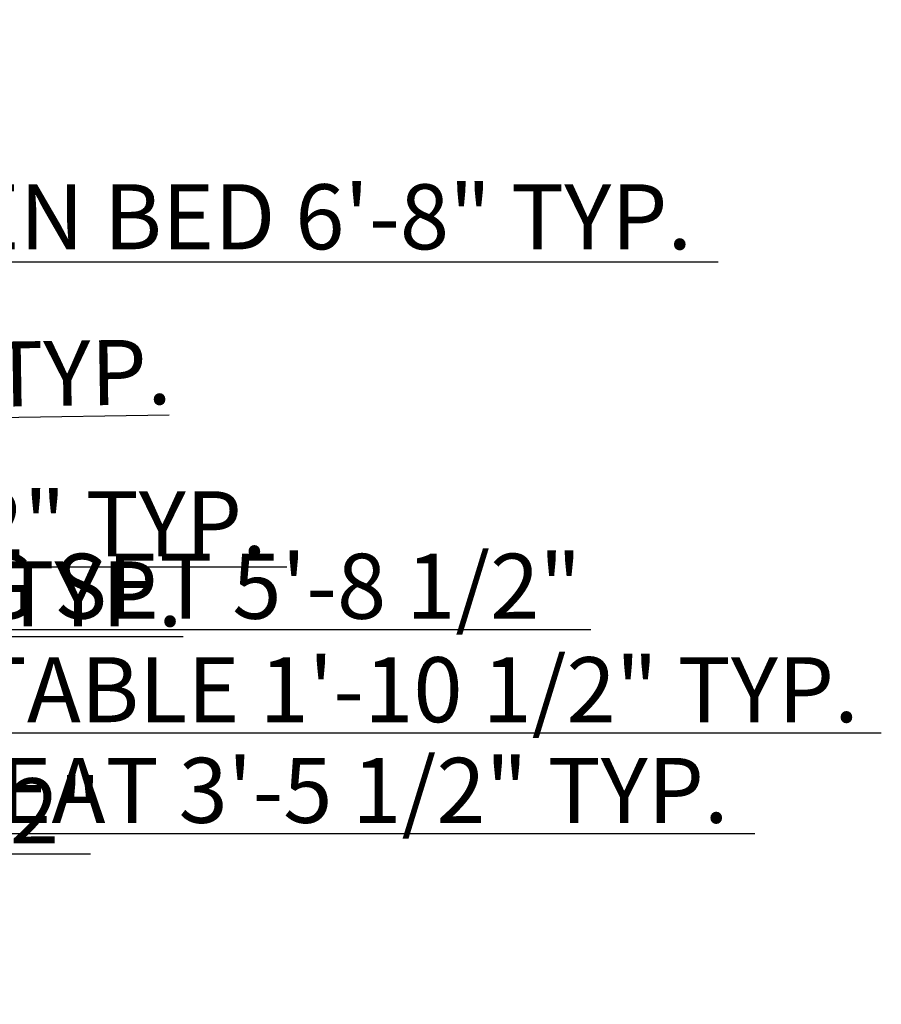
# Model space of a CAD drawing. Units: inches. Extents: x 2901 to 21549, y 2042 to 3828.
# Tile 10 of 10: x 3774 to 4251, y 2948 to 3493. Entities that reach past the tile are written whole.
import ezdxf

# ---------------------------------------------------------------- set-up
doc = ezdxf.new("R2010")
doc.units = ezdxf.units.IN
doc.layers.get('Defpoints').update_dxf_attribs({"color": 1})
doc.layers.add('A-ANNO-DIMS', color=2, linetype='Continuous', lineweight=18)
doc.styles.get("Standard").update_dxf_attribs({"font": 'arial.ttf'})
doc.dimstyles.new('ISO-25', dxfattribs={"dimtxt": 36, "dimasz": 5, "dimexe": 1.25, "dimexo": 0.625, "dimtad": 1, "dimdec": 0, "dimlunit": 3, "dimtxsty": 'Standard', "dimcen": 2.5, "dimadec": 0, "dimazin": 0, "dimtfac": 1, "dimtdec": 0, "dimtmove": 0, "dimatfit": 3, "dimfxl": 1, "dimarcsym": 0})

# ---------------------------------------------------------------- blocks, each defined once
blk = doc.blocks.new('*D37')
at = {"layer": 'A-ANNO-DIMS', "color": 0, "lineweight": -2, "transparency": 16777216}
for p, q in [((3620.07, 3151.24), (3615.07, 3151.24)), ((3625.07, 3156.01), (3625.07, 3149.99)), ((3625.07, 3151.24), (3634.07, 3151.24)), ((3634.07, 3156.01), (3634.07, 3149.99)), ((3639.07, 3151.24), (3864.76, 3151.24))]:
    blk.add_line(p, q, dxfattribs=at)
at = {"layer": 'A-ANNO-DIMS', "color": 0, "transparency": 16777216}
for points in [[(3620.07, 3152.07), (3620.07, 3150.41), (3625.07, 3151.24)], [(3639.07, 3152.07), (3639.07, 3150.41), (3634.07, 3151.24)]]:
    blk.add_solid(points, dxfattribs=at)
at = {"layer": 'Defpoints', "color": 0, "transparency": 16777216}
for p in [(3625.07, 3156.64), (3634.07, 3156.64), (3634.07, 3151.24)]:
    blk.add_point(p, dxfattribs=at)
at = {"layer": 'A-ANNO-DIMS', "color": 0, "transparency": 16777216, "insert": (3754.41, 3170.24), "char_height": 36, "attachment_point": 5}
blk.add_mtext('0\'-9" TYP.', dxfattribs=at)
blk = doc.blocks.new('*D38')
at = {"layer": 'A-ANNO-DIMS', "color": 0, "lineweight": -2, "transparency": 16777216}
for p, q in [((3343.07, 3191.34), (3343.07, 3188.58)), ((3348.07, 3189.83), (3352.29, 3189.83)), ((3357.29, 3191.34), (3357.29, 3188.58)), ((3357.29, 3189.83), (3922.11, 3189.83))]:
    blk.add_line(p, q, dxfattribs=at)
at = {"layer": 'A-ANNO-DIMS', "color": 0, "transparency": 16777216}
for points in [[(3348.07, 3190.67), (3348.07, 3189), (3343.07, 3189.83)], [(3352.29, 3190.67), (3352.29, 3189), (3357.29, 3189.83)]]:
    blk.add_solid(points, dxfattribs=at)
at = {"layer": 'Defpoints', "color": 0, "transparency": 16777216}
for p in [(3343.07, 3191.97), (3357.29, 3191.97), (3357.29, 3189.83)]:
    blk.add_point(p, dxfattribs=at)
at = {"layer": 'A-ANNO-DIMS', "color": 0, "transparency": 16777216, "insert": (3642.2, 3209.07), "char_height": 36, "attachment_point": 5}
blk.add_mtext('NIGHTSTAND 1\'-2" TYP.', dxfattribs=at)
blk = doc.blocks.new('*D43')
at = {"layer": 'A-ANNO-DIMS', "color": 0, "lineweight": -2, "transparency": 16777216}
for p, q in [((3550.8, 3269.4), (3856.95, 3274.04)), ((3536.1, 3267.11), (3536.05, 3270.42)), ((3541.07, 3269.25), (3545.8, 3269.32)), ((3550.83, 3267.33), (3550.78, 3270.65))]:
    blk.add_line(p, q, dxfattribs=at)
at = {"layer": 'A-ANNO-DIMS', "color": 0, "transparency": 16777216}
for points in [[(3541.06, 3270.08), (3541.09, 3268.42), (3536.07, 3269.17)], [(3545.78, 3270.16), (3545.81, 3268.49), (3550.8, 3269.4)]]:
    blk.add_solid(points, dxfattribs=at)
at = {"layer": 'Defpoints', "color": 0, "transparency": 16777216}
for p in [(3536.11, 3266.48), (3550.8, 3269.4), (3550.84, 3266.71)]:
    blk.add_point(p, dxfattribs=at)
at = {"layer": 'A-ANNO-DIMS', "color": 0, "transparency": 16777216, "insert": (3706.08, 3290.99), "char_height": 36, "attachment_point": 5, "rotation": 0.8679}
blk.add_mtext('1\'-2 1/2" TYP.', dxfattribs=at)
blk = doc.blocks.new('*D46')
at = {"layer": 'A-ANNO-DIMS', "color": 0, "lineweight": -2, "transparency": 16777216}
for p, q in [((3545.07, 3370.05), (3545.07, 3357.42)), ((3625.07, 3370.05), (3625.07, 3357.42)), ((3550.07, 3358.67), (3620.07, 3358.67)), ((3625.07, 3358.67), (4160.88, 3358.67))]:
    blk.add_line(p, q, dxfattribs=at)
at = {"layer": 'A-ANNO-DIMS', "color": 0, "transparency": 16777216}
for points in [[(3550.07, 3359.51), (3550.07, 3357.84), (3545.07, 3358.67)], [(3620.07, 3359.51), (3620.07, 3357.84), (3625.07, 3358.67)]]:
    blk.add_solid(points, dxfattribs=at)
at = {"layer": 'Defpoints', "color": 0, "transparency": 16777216}
for p in [(3545.07, 3370.67), (3625.07, 3370.67), (3625.07, 3358.67)]:
    blk.add_point(p, dxfattribs=at)
at = {"layer": 'A-ANNO-DIMS', "color": 0, "transparency": 16777216, "insert": (3895.48, 3379.02), "char_height": 36, "attachment_point": 5}
blk.add_mtext('QUEEN BED 6\'-8" TYP.', dxfattribs=at)
blk = doc.blocks.new('*D48')
at = {"layer": 'A-ANNO-DIMS', "color": 0, "lineweight": -2, "transparency": 16777216}
for p, q in [((3552.33, 3036.58), (3552.33, 3043.43)), ((3557.33, 3042.18), (3588.77, 3042.18)), ((3593.77, 3036.58), (3593.77, 3043.43)), ((3593.77, 3042.18), (4181.25, 3042.18))]:
    blk.add_line(p, q, dxfattribs=at)
at = {"layer": 'A-ANNO-DIMS', "color": 0, "transparency": 16777216}
for points in [[(3557.33, 3043.01), (3557.33, 3041.34), (3552.33, 3042.18)], [(3588.77, 3043.01), (3588.77, 3041.34), (3593.77, 3042.18)]]:
    blk.add_solid(points, dxfattribs=at)
at = {"layer": 'Defpoints', "color": 0, "transparency": 16777216}
for p in [(3593.77, 3042.18), (3552.33, 3035.96), (3593.77, 3035.96)]:
    blk.add_point(p, dxfattribs=at)
at = {"layer": 'A-ANNO-DIMS', "color": 0, "transparency": 16777216, "insert": (3890.01, 3061.44), "char_height": 36, "attachment_point": 5}
blk.add_mtext('LOVESEAT 3\'-5 1/2" TYP.', dxfattribs=at)
blk = doc.blocks.new('*D50')
at = {"layer": 'A-ANNO-DIMS', "color": 0, "lineweight": -2, "transparency": 16777216}
for p, q in [((3599.61, 3100.68), (3599.61, 3096.69)), ((3604.61, 3097.94), (3617.08, 3097.94)), ((3622.08, 3100.68), (3622.08, 3096.69)), ((3622.08, 3097.94), (4251.18, 3097.94))]:
    blk.add_line(p, q, dxfattribs=at)
at = {"layer": 'A-ANNO-DIMS', "color": 0, "transparency": 16777216}
for points in [[(3604.61, 3098.77), (3604.61, 3097.1), (3599.61, 3097.94)], [(3617.08, 3098.77), (3617.08, 3097.1), (3622.08, 3097.94)]]:
    blk.add_solid(points, dxfattribs=at)
at = {"layer": 'Defpoints', "color": 0, "transparency": 16777216}
for p in [(3599.61, 3101.31), (3622.08, 3101.31), (3622.08, 3097.94)]:
    blk.add_point(p, dxfattribs=at)
at = {"layer": 'A-ANNO-DIMS', "color": 0, "transparency": 16777216, "insert": (3939.13, 3117.18), "char_height": 36, "attachment_point": 5}
blk.add_mtext('END TABLE 1\'-10 1/2" TYP.', dxfattribs=at)
blk = doc.blocks.new('*D54')
at = {"layer": 'A-ANNO-DIMS', "color": 0, "lineweight": -2, "transparency": 16777216}
for p, q in [((3536.12, 3164.87), (3536.12, 3153.97)), ((3604.61, 3164.87), (3604.61, 3153.97)), ((3541.12, 3155.22), (3599.61, 3155.22)), ((3604.61, 3155.22), (4090.43, 3155.22))]:
    blk.add_line(p, q, dxfattribs=at)
at = {"layer": 'A-ANNO-DIMS', "color": 0, "transparency": 16777216}
for points in [[(3541.12, 3156.05), (3541.12, 3154.38), (3536.12, 3155.22)], [(3599.61, 3156.05), (3599.61, 3154.38), (3604.61, 3155.22)]]:
    blk.add_solid(points, dxfattribs=at)
at = {"layer": 'Defpoints', "color": 0, "transparency": 16777216}
for p in [(3536.12, 3165.49), (3604.61, 3165.49), (3604.61, 3155.22)]:
    blk.add_point(p, dxfattribs=at)
at = {"layer": 'A-ANNO-DIMS', "color": 0, "transparency": 16777216, "insert": (3850.02, 3174.46), "char_height": 36, "attachment_point": 5}
blk.add_mtext('DINING SET 5\'-8 1/2"', dxfattribs=at)
blk = doc.blocks.new('*D57')
at = {"layer": 'A-ANNO-DIMS', "color": 0, "lineweight": -2, "transparency": 16777216}
for p, q in [((3601.59, 3038.97), (3601.59, 3029.64)), ((3626.91, 3038.97), (3626.91, 3029.64)), ((3606.59, 3030.89), (3621.91, 3030.89)), ((3626.91, 3030.89), (3813.36, 3030.89))]:
    blk.add_line(p, q, dxfattribs=at)
at = {"layer": 'A-ANNO-DIMS', "color": 0, "transparency": 16777216}
for points in [[(3606.59, 3031.73), (3606.59, 3030.06), (3601.59, 3030.89)], [(3621.91, 3031.73), (3621.91, 3030.06), (3626.91, 3030.89)]]:
    blk.add_solid(points, dxfattribs=at)
at = {"layer": 'Defpoints', "color": 0, "transparency": 16777216}
for p in [(3601.59, 3039.6), (3626.91, 3039.6), (3626.91, 3030.89)]:
    blk.add_point(p, dxfattribs=at)
at = {"layer": 'A-ANNO-DIMS', "color": 0, "transparency": 16777216, "insert": (3722.63, 3050.13), "char_height": 36, "attachment_point": 5}
blk.add_mtext('2\'-1 1/2"', dxfattribs=at)

msp = doc.modelspace()

# ---------------------------------------------------------------- dimensions: what is measured, and where the dimension line sits
at = {"layer": 'A-ANNO-DIMS'}
for base, p1, p2, text, picture, middle in [((3625.07, 3358.67), (3545.07, 3370.67), (3625.07, 3370.67), 'QUEEN BED <> TYP.', '*D46', (3895.48, 3379.02)), ((3357.29, 3189.83), (3343.07, 3191.97), (3357.29, 3191.97), 'NIGHTSTAND <> TYP.', '*D38', (3642.2, 3209.07)), ((3604.61, 3155.22), (3536.12, 3165.49), (3604.61, 3165.49), 'DINING SET <>', '*D54', (3850.02, 3174.46)), ((3622.08, 3097.94), (3599.61, 3101.31), (3622.08, 3101.31), 'END TABLE <> TYP.', '*D50', (3939.13, 3117.18)), ((3634.07, 3151.24), (3625.07, 3156.64), (3634.07, 3156.64), '<> TYP.', '*D37', (3754.41, 3170.24)), ((3593.77, 3042.18), (3552.33, 3035.96), (3593.77, 3035.96), 'LOVESEAT <> TYP.', '*D48', (3890.01, 3061.44))]:
    dim = msp.add_linear_dim(base=base, p1=p1, p2=p2, text=text, dimstyle='ISO-25', override={"dimdec": 1, "dimlfac": 1, "dimrnd": 0, "dimzin": 1, "dimdsep": 46, "dimlunit": 4, "dimfrac": 2}, dxfattribs=at)
    dim.commit()
    dim.dimension.update_dxf_attribs({"geometry": picture, "text_midpoint": middle})
dim = msp.add_linear_dim(base=(3550.8, 3269.4), p1=(3536.11, 3266.48), p2=(3550.84, 3266.71), angle=0.8679, text='<> TYP.', dimstyle='ISO-25', override={"dimdec": 1, "dimlfac": 1, "dimrnd": 0, "dimzin": 1, "dimdsep": 46, "dimlunit": 4, "dimfrac": 2}, dxfattribs=at)
dim.commit()
dim.dimension.update_dxf_attribs({"geometry": '*D43', "text_midpoint": (3706.08, 3290.99)})
dim = msp.add_linear_dim(base=(3626.91, 3030.89), p1=(3601.59, 3039.6), p2=(3626.91, 3039.6), dimstyle='ISO-25', override={"dimdec": 1, "dimlfac": 1, "dimrnd": 0, "dimzin": 1, "dimdsep": 46, "dimlunit": 4, "dimfrac": 2}, dxfattribs=at)
dim.commit()
dim.dimension.update_dxf_attribs({"geometry": '*D57', "text_midpoint": (3722.63, 3050.13)})

doc.saveas('drawing.dxf')
